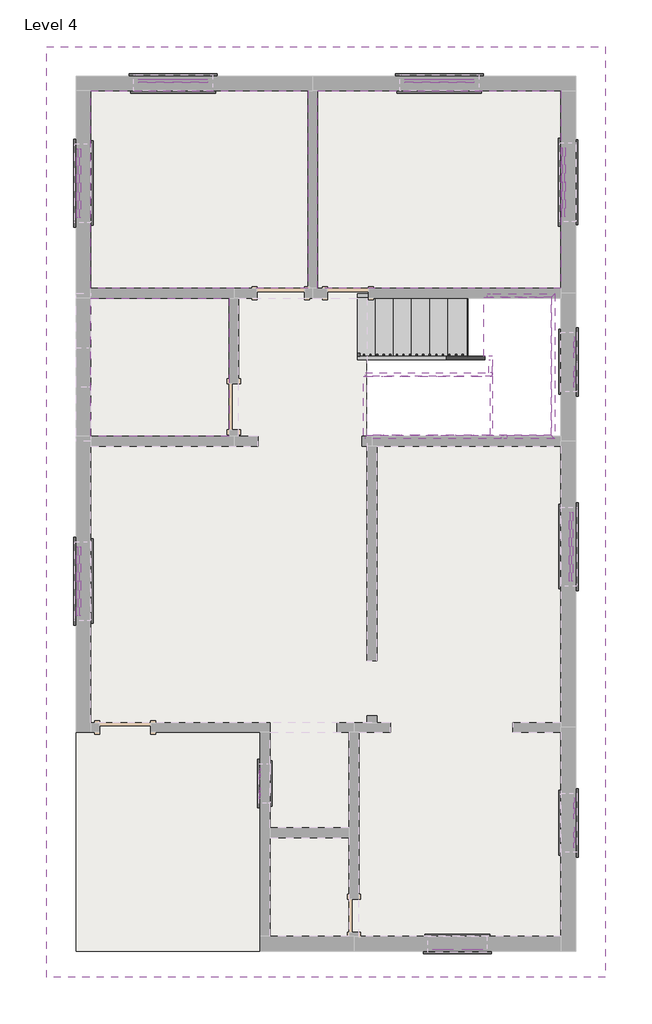
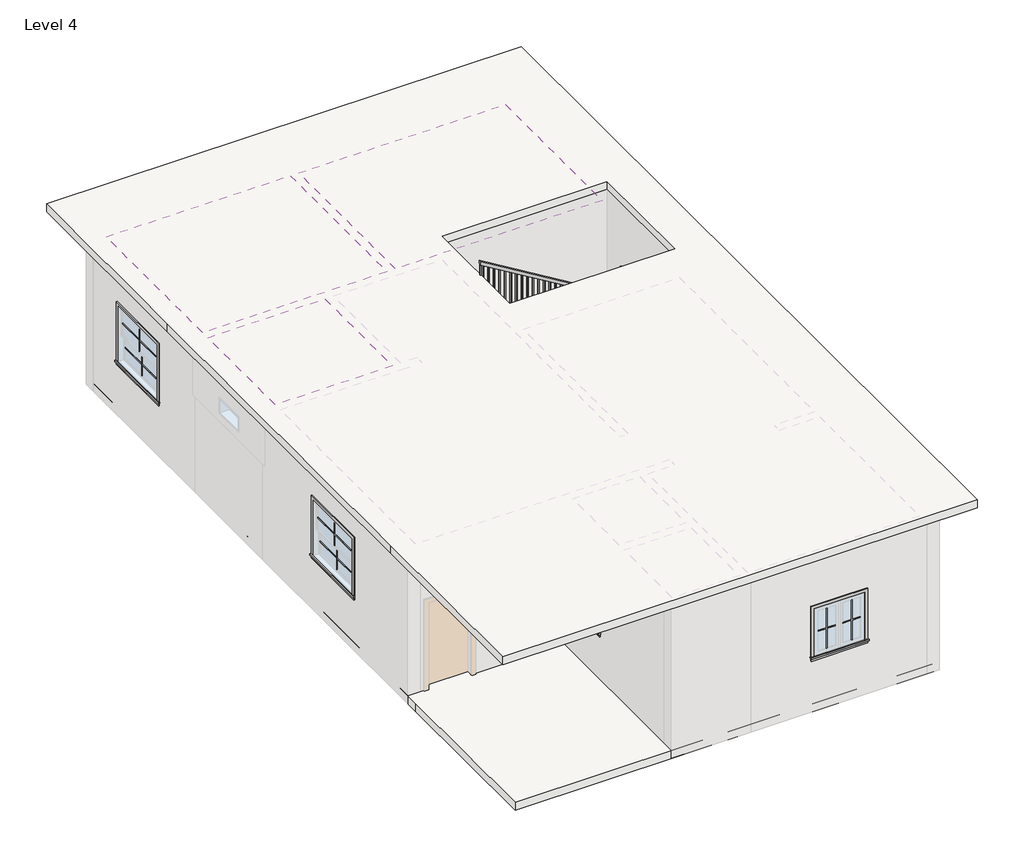
# One storey, part 2 of 2: 40 proxies, 8 members, 3 coverings, 3 slabs, 2 stair flights, 1 railing.
"""IFC4 building model written with IfcOpenShell, lengths in millimetres."""

from ifc_helpers import new_model, si_unit, frame, origin, place, context, project, spatial, polyline, outline, extrude, faceted_brep, transform, mapped, element, save
from components import muntin_pattern_2x2_muntin_pattern_2x2_8b3f23e7, muntin_pattern_2x2_muntin_pattern_2x2_5e52a1c6, muntin_pattern_2x2_muntin_pattern_2x2_d1c6e638, muntin_pattern_2x2_muntin_pattern_2x2_37b95fb2, muntin_pattern_2x2_muntin_pattern_2x2_53152e2c, muntin_pattern_2x2_muntin_pattern_2x2_e8f3e573, trim_window_exterior_flat_with_sill_f44f30ad, trim_window_exterior_flat_with_sill_e2e7eb1d, trim_window_exterior_flat_with_sill_84e24481, trim_window_exterior_flat_with_sill_a665a915, trim_window_interior_flat_picture_frame_1dce1945, trim_window_interior_flat_picture_frame_a40cb921, trim_window_interior_flat_picture_frame_28d4e5dc, trim_window_interior_flat_picture_frame_d485c387, non_monolithic_landing_28d2b2aa, stair_flight_33a07897, stair_flight_2b211656

model = new_model("IFC4")

# Units and contexts
model_context = context("Model", 3, world=origin())
ifc_project = project(units=[si_unit("LENGTHUNIT", "METRE", prefix="MILLI")], contexts=[model_context])

# Site, building, storey
site = spatial("IfcSite", under=ifc_project)
building = spatial("IfcBuilding", under=site)
storey = spatial("IfcBuildingStorey", under=building, Name="Level 4", Elevation=9601.2)

# Proxies
placement = place(None, origin())
muntin_pattern_2x2_muntin_pattern_2x2_shape = muntin_pattern_2x2_muntin_pattern_2x2_8b3f23e7(model_context)
element("IfcBuildingElementProxy", 1, Name="Muntin Pattern_2x2 : Muntin Pattern_2x2", ObjectType="Muntin Pattern_2x2 : Muntin Pattern_2x2", at=placement, inside=storey, context=model_context, shape_type="MappedRepresentation", body=[
    mapped(muntin_pattern_2x2_muntin_pattern_2x2_shape, transform((-5865.439062, 5032.1857363, 11376.025), x_axis=(0.0, 1.0, 0.0), y_axis=(-1.0, 0.0, 0.0), z_axis=(0.0, 0.0, 1.0))),
])
element("IfcBuildingElementProxy", 2, Name="Muntin Pattern_2x2 : Muntin Pattern_2x2", ObjectType="Muntin Pattern_2x2 : Muntin Pattern_2x2", at=placement, inside=storey, context=model_context, shape_type="MappedRepresentation", body=[
    mapped(muntin_pattern_2x2_muntin_pattern_2x2_shape, transform((-5820.989062, 5032.1857363, 10896.6), x_axis=(0.0, 1.0, 0.0), y_axis=(-1.0, 0.0, 0.0), z_axis=(0.0, 0.0, 1.0))),
])
element("IfcBuildingElementProxy", 3, Name="Muntin Pattern_2x2 : Muntin Pattern_2x2", ObjectType="Muntin Pattern_2x2 : Muntin Pattern_2x2", at=placement, inside=storey, context=model_context, shape_type="MappedRepresentation", body=[
    mapped(muntin_pattern_2x2_muntin_pattern_2x2_shape, transform((1786.310938, -581.2142637, 11376.025), x_axis=(0.0, -1.0, 0.0), y_axis=(1.0, 0.0, 0.0), z_axis=(0.0, 0.0, 1.0))),
])
element("IfcBuildingElementProxy", 4, Name="Muntin Pattern_2x2 : Muntin Pattern_2x2", ObjectType="Muntin Pattern_2x2 : Muntin Pattern_2x2", at=placement, inside=storey, context=model_context, shape_type="MappedRepresentation", body=[
    mapped(muntin_pattern_2x2_muntin_pattern_2x2_shape, transform((1741.860938, -581.2142637, 10896.6), x_axis=(0.0, -1.0, 0.0), y_axis=(1.0, 0.0, 0.0), z_axis=(0.0, 0.0, 1.0))),
])
element("IfcBuildingElementProxy", 5, Name="Muntin Pattern_2x2 : Muntin Pattern_2x2", ObjectType="Muntin Pattern_2x2 : Muntin Pattern_2x2", at=placement, inside=storey, context=model_context, shape_type="MappedRepresentation", body=[
    mapped(muntin_pattern_2x2_muntin_pattern_2x2_shape, transform((-5865.439062, -1114.6142637, 11376.025), x_axis=(0.0, 1.0, 0.0), y_axis=(-1.0, 0.0, 0.0), z_axis=(0.0, 0.0, 1.0))),
])
element("IfcBuildingElementProxy", 6, Name="Muntin Pattern_2x2 : Muntin Pattern_2x2", ObjectType="Muntin Pattern_2x2 : Muntin Pattern_2x2", at=placement, inside=storey, context=model_context, shape_type="MappedRepresentation", body=[
    mapped(muntin_pattern_2x2_muntin_pattern_2x2_shape, transform((-5820.989062, -1114.6142637, 10896.6), x_axis=(0.0, 1.0, 0.0), y_axis=(-1.0, 0.0, 0.0), z_axis=(0.0, 0.0, 1.0))),
])
muntin_pattern_2x2_muntin_pattern_2x2_2_shape = muntin_pattern_2x2_muntin_pattern_2x2_5e52a1c6(model_context)
element("IfcBuildingElementProxy", 7, Name="Muntin Pattern_2x2 : Muntin Pattern_2x2", ObjectType="Muntin Pattern_2x2 : Muntin Pattern_2x2", at=placement, inside=storey, context=model_context, shape_type="MappedRepresentation", body=[
    mapped(muntin_pattern_2x2_muntin_pattern_2x2_2_shape, transform((-4401.764062, 6648.2607363, 11376.025), x_axis=(-1.0, 0.0, 0.0), y_axis=(0.0, -1.0, 0.0), z_axis=(0.0, 0.0, 1.0))),
])
element("IfcBuildingElementProxy", 8, Name="Muntin Pattern_2x2 : Muntin Pattern_2x2", ObjectType="Muntin Pattern_2x2 : Muntin Pattern_2x2", at=placement, inside=storey, context=model_context, shape_type="MappedRepresentation", body=[
    mapped(muntin_pattern_2x2_muntin_pattern_2x2_2_shape, transform((-4401.764062, 6603.8107363, 10896.6), x_axis=(-1.0, 0.0, 0.0), y_axis=(0.0, -1.0, 0.0), z_axis=(0.0, 0.0, 1.0))),
])
element("IfcBuildingElementProxy", 9, Name="Muntin Pattern_2x2 : Muntin Pattern_2x2", ObjectType="Muntin Pattern_2x2 : Muntin Pattern_2x2", at=placement, inside=storey, context=model_context, shape_type="MappedRepresentation", body=[
    mapped(muntin_pattern_2x2_muntin_pattern_2x2_2_shape, transform((-286.964062, 6648.2607363, 11376.025), x_axis=(-1.0, 0.0, 0.0), y_axis=(0.0, -1.0, 0.0), z_axis=(0.0, 0.0, 1.0))),
])
element("IfcBuildingElementProxy", 10, Name="Muntin Pattern_2x2 : Muntin Pattern_2x2", ObjectType="Muntin Pattern_2x2 : Muntin Pattern_2x2", at=placement, inside=storey, context=model_context, shape_type="MappedRepresentation", body=[
    mapped(muntin_pattern_2x2_muntin_pattern_2x2_2_shape, transform((-286.964062, 6603.8107363, 10896.6), x_axis=(-1.0, 0.0, 0.0), y_axis=(0.0, -1.0, 0.0), z_axis=(0.0, 0.0, 1.0))),
])
element("IfcBuildingElementProxy", 11, Name="Muntin Pattern_2x2 : Muntin Pattern_2x2", ObjectType="Muntin Pattern_2x2 : Muntin Pattern_2x2", at=placement, inside=storey, context=model_context, shape_type="MappedRepresentation", body=[
    mapped(muntin_pattern_2x2_muntin_pattern_2x2_2_shape, transform((1627.560938, 5044.8857363, 11376.025), x_axis=(0.0, -1.0, 0.0), y_axis=(1.0, 0.0, 0.0), z_axis=(0.0, 0.0, 1.0))),
])
element("IfcBuildingElementProxy", 12, Name="Muntin Pattern_2x2 : Muntin Pattern_2x2", ObjectType="Muntin Pattern_2x2 : Muntin Pattern_2x2", at=placement, inside=storey, context=model_context, shape_type="MappedRepresentation", body=[
    mapped(muntin_pattern_2x2_muntin_pattern_2x2_2_shape, transform((1672.010938, 5044.8857363, 10896.6), x_axis=(0.0, -1.0, 0.0), y_axis=(1.0, 0.0, 0.0), z_axis=(0.0, 0.0, 1.0))),
])
muntin_pattern_2x2_muntin_pattern_2x2_3_shape = muntin_pattern_2x2_muntin_pattern_2x2_d1c6e638(model_context)
element("IfcBuildingElementProxy", 13, Name="Muntin Pattern_2x2 : Muntin Pattern_2x2", ObjectType="Muntin Pattern_2x2 : Muntin Pattern_2x2", at=placement, inside=storey, context=model_context, shape_type="MappedRepresentation", body=[
    mapped(muntin_pattern_2x2_muntin_pattern_2x2_3_shape, transform((1811.710938, -4621.4017637, 10890.25), x_axis=(0.0, -1.0, 0.0), y_axis=(1.0, 0.0, 0.0), z_axis=(0.0, 0.0, 1.0))),
])
element("IfcBuildingElementProxy", 14, Name="Muntin Pattern_2x2 : Muntin Pattern_2x2", ObjectType="Muntin Pattern_2x2 : Muntin Pattern_2x2", at=placement, inside=storey, context=model_context, shape_type="MappedRepresentation", body=[
    mapped(muntin_pattern_2x2_muntin_pattern_2x2_3_shape, transform((219.448438, -6820.0892637, 10890.25), x_axis=(-1.0, 0.0, 0.0), y_axis=(0.0, -1.0, 0.0), z_axis=(0.0, 0.0, 1.0))),
])
element("IfcBuildingElementProxy", 15, Name="Muntin Pattern_2x2 : Muntin Pattern_2x2", ObjectType="Muntin Pattern_2x2 : Muntin Pattern_2x2", at=placement, inside=storey, context=model_context, shape_type="MappedRepresentation", body=[
    mapped(muntin_pattern_2x2_muntin_pattern_2x2_3_shape, transform((1811.710938, 2496.9482363, 10890.25), x_axis=(0.0, -1.0, 0.0), y_axis=(1.0, 0.0, 0.0), z_axis=(0.0, 0.0, 1.0))),
])
muntin_pattern_2x2_muntin_pattern_2x2_4_shape = muntin_pattern_2x2_muntin_pattern_2x2_37b95fb2(model_context)
element("IfcBuildingElementProxy", 16, Name="Muntin Pattern_2x2 : Muntin Pattern_2x2", ObjectType="Muntin Pattern_2x2 : Muntin Pattern_2x2", at=placement, inside=storey, context=model_context, shape_type="MappedRepresentation", body=[
    mapped(muntin_pattern_2x2_muntin_pattern_2x2_4_shape, transform((1811.710938, -5075.4267637, 10890.25), x_axis=(0.0, 1.0, 0.0), y_axis=(-1.0, 0.0, 0.0), z_axis=(0.0, 0.0, 1.0))),
])
element("IfcBuildingElementProxy", 17, Name="Muntin Pattern_2x2 : Muntin Pattern_2x2", ObjectType="Muntin Pattern_2x2 : Muntin Pattern_2x2", at=placement, inside=storey, context=model_context, shape_type="MappedRepresentation", body=[
    mapped(muntin_pattern_2x2_muntin_pattern_2x2_4_shape, transform((-234.576562, -6820.0892637, 10890.25), x_axis=(1.0, 0.0, 0.0), y_axis=(0.0, 1.0, 0.0), z_axis=(0.0, 0.0, 1.0))),
])
element("IfcBuildingElementProxy", 18, Name="Muntin Pattern_2x2 : Muntin Pattern_2x2", ObjectType="Muntin Pattern_2x2 : Muntin Pattern_2x2", at=placement, inside=storey, context=model_context, shape_type="MappedRepresentation", body=[
    mapped(muntin_pattern_2x2_muntin_pattern_2x2_4_shape, transform((1811.710938, 2042.9232363, 10890.25), x_axis=(0.0, 1.0, 0.0), y_axis=(-1.0, 0.0, 0.0), z_axis=(0.0, 0.0, 1.0))),
])
muntin_pattern_2x2_muntin_pattern_2x2_5_shape = muntin_pattern_2x2_muntin_pattern_2x2_53152e2c(model_context)
element("IfcBuildingElementProxy", 19, Name="Muntin Pattern_2x2 : Muntin Pattern_2x2", ObjectType="Muntin Pattern_2x2 : Muntin Pattern_2x2", at=placement, inside=storey, context=model_context, shape_type="MappedRepresentation", body=[
    mapped(muntin_pattern_2x2_muntin_pattern_2x2_5_shape, transform((-3046.039062, -4389.6267637, 10890.25), x_axis=(0.0, 1.0, 0.0), y_axis=(-1.0, 0.0, 0.0), z_axis=(0.0, 0.0, 1.0))),
])
muntin_pattern_2x2_muntin_pattern_2x2_6_shape = muntin_pattern_2x2_muntin_pattern_2x2_e8f3e573(model_context)
element("IfcBuildingElementProxy", 20, Name="Muntin Pattern_2x2 : Muntin Pattern_2x2", ObjectType="Muntin Pattern_2x2 : Muntin Pattern_2x2", at=placement, inside=storey, context=model_context, shape_type="MappedRepresentation", body=[
    mapped(muntin_pattern_2x2_muntin_pattern_2x2_6_shape, transform((-3046.039062, -4088.0017637, 10890.25), x_axis=(0.0, -1.0, 0.0), y_axis=(1.0, 0.0, 0.0), z_axis=(0.0, 0.0, 1.0))),
])
trim_window_exterior_flat_with_sill_shape = trim_window_exterior_flat_with_sill_f44f30ad(model_context)
element("IfcBuildingElementProxy", 21, Name="Trim-Window-Exterior-Flat : with Sill", ObjectType="Trim-Window-Exterior-Flat : with Sill", at=placement, inside=storey, context=model_context, shape_type="MappedRepresentation", body=[
    mapped(trim_window_exterior_flat_with_sill_shape, transform((-5900.364062, 5032.1857363, 11887.2), x_axis=(0.0, -1.0, 0.0), y_axis=(0.0, 0.0, 1.0), z_axis=(-1.0, 0.0, 0.0))),
])
element("IfcBuildingElementProxy", 22, Name="Trim-Window-Exterior-Flat : with Sill", ObjectType="Trim-Window-Exterior-Flat : with Sill", at=placement, inside=storey, context=model_context, shape_type="MappedRepresentation", body=[
    mapped(trim_window_exterior_flat_with_sill_shape, transform((1821.235938, -581.2142637, 11887.2), x_axis=(0.0, 1.0, 0.0), y_axis=(0.0, 0.0, 1.0), z_axis=(1.0, 0.0, 0.0))),
])
element("IfcBuildingElementProxy", 23, Name="Trim-Window-Exterior-Flat : with Sill", ObjectType="Trim-Window-Exterior-Flat : with Sill", at=placement, inside=storey, context=model_context, shape_type="MappedRepresentation", body=[
    mapped(trim_window_exterior_flat_with_sill_shape, transform((-5900.364062, -1114.6142637, 11887.2), x_axis=(0.0, -1.0, 0.0), y_axis=(0.0, 0.0, 1.0), z_axis=(-1.0, 0.0, 0.0))),
])
trim_window_exterior_flat_with_sill_2_shape = trim_window_exterior_flat_with_sill_e2e7eb1d(model_context)
element("IfcBuildingElementProxy", 24, Name="Trim-Window-Exterior-Flat : with Sill", ObjectType="Trim-Window-Exterior-Flat : with Sill", at=placement, inside=storey, context=model_context, shape_type="MappedRepresentation", body=[
    mapped(trim_window_exterior_flat_with_sill_2_shape, transform((-4401.764062, 6683.1857363, 11887.2), x_axis=(1.0, 0.0, 0.0), y_axis=(0.0, 0.0, -1.0), z_axis=(0.0, 1.0, 0.0))),
])
element("IfcBuildingElementProxy", 25, Name="Trim-Window-Exterior-Flat : with Sill", ObjectType="Trim-Window-Exterior-Flat : with Sill", at=placement, inside=storey, context=model_context, shape_type="MappedRepresentation", body=[
    mapped(trim_window_exterior_flat_with_sill_2_shape, transform((-286.964062, 6683.1857363, 11887.2), x_axis=(1.0, 0.0, 0.0), y_axis=(0.0, 0.0, -1.0), z_axis=(0.0, 1.0, 0.0))),
])
element("IfcBuildingElementProxy", 26, Name="Trim-Window-Exterior-Flat : with Sill", ObjectType="Trim-Window-Exterior-Flat : with Sill", at=placement, inside=storey, context=model_context, shape_type="MappedRepresentation", body=[
    mapped(trim_window_exterior_flat_with_sill_2_shape, transform((1592.635938, 5044.8857363, 11887.2), x_axis=(0.0, 1.0, 0.0), y_axis=(0.0, 0.0, -1.0), z_axis=(-1.0, 0.0, 0.0))),
])
trim_window_exterior_flat_with_sill_3_shape = trim_window_exterior_flat_with_sill_84e24481(model_context)
element("IfcBuildingElementProxy", 27, Name="Trim-Window-Exterior-Flat : with Sill", ObjectType="Trim-Window-Exterior-Flat : with Sill", at=placement, inside=storey, context=model_context, shape_type="MappedRepresentation", body=[
    mapped(trim_window_exterior_flat_with_sill_3_shape, transform((1821.235938, -4848.4142637, 11734.8), x_axis=(0.0, 1.0, 0.0), y_axis=(0.0, 0.0, 1.0), z_axis=(1.0, 0.0, 0.0))),
])
element("IfcBuildingElementProxy", 28, Name="Trim-Window-Exterior-Flat : with Sill", ObjectType="Trim-Window-Exterior-Flat : with Sill", at=placement, inside=storey, context=model_context, shape_type="MappedRepresentation", body=[
    mapped(trim_window_exterior_flat_with_sill_3_shape, transform((-7.564062, -6829.6142637, 11734.8), x_axis=(1.0, 0.0, 0.0), y_axis=(0.0, 0.0, 1.0), z_axis=(0.0, -1.0, 0.0))),
])
element("IfcBuildingElementProxy", 29, Name="Trim-Window-Exterior-Flat : with Sill", ObjectType="Trim-Window-Exterior-Flat : with Sill", at=placement, inside=storey, context=model_context, shape_type="MappedRepresentation", body=[
    mapped(trim_window_exterior_flat_with_sill_3_shape, transform((1821.235938, 2269.9357363, 11734.8), x_axis=(0.0, 1.0, 0.0), y_axis=(0.0, 0.0, 1.0), z_axis=(1.0, 0.0, 0.0))),
])
trim_window_exterior_flat_with_sill_4_shape = trim_window_exterior_flat_with_sill_a665a915(model_context)
element("IfcBuildingElementProxy", 30, Name="Trim-Window-Exterior-Flat : with Sill", ObjectType="Trim-Window-Exterior-Flat : with Sill", at=placement, inside=storey, context=model_context, shape_type="MappedRepresentation", body=[
    mapped(trim_window_exterior_flat_with_sill_4_shape, transform((-3055.564062, -4238.8142637, 11734.8), x_axis=(0.0, -1.0, 0.0), y_axis=(0.0, 0.0, 1.0), z_axis=(-1.0, 0.0, 0.0))),
])
trim_window_interior_flat_picture_frame_shape = trim_window_interior_flat_picture_frame_1dce1945(model_context)
element("IfcBuildingElementProxy", 31, Name="Trim-Window-Interior-Flat : Picture Frame", ObjectType="Trim-Window-Interior-Flat : Picture Frame", at=placement, inside=storey, context=model_context, shape_type="MappedRepresentation", body=[
    mapped(trim_window_interior_flat_picture_frame_shape, transform((-5671.764062, 5032.1857363, 11887.2), x_axis=(0.0, 1.0, 0.0), y_axis=(0.0, 0.0, 1.0), z_axis=(1.0, 0.0, 0.0))),
])
element("IfcBuildingElementProxy", 32, Name="Trim-Window-Interior-Flat : Picture Frame", ObjectType="Trim-Window-Interior-Flat : Picture Frame", at=placement, inside=storey, context=model_context, shape_type="MappedRepresentation", body=[
    mapped(trim_window_interior_flat_picture_frame_shape, transform((1592.635938, -581.2142637, 11887.2), x_axis=(0.0, -1.0, 0.0), y_axis=(0.0, 0.0, 1.0), z_axis=(-1.0, 0.0, 0.0))),
])
element("IfcBuildingElementProxy", 33, Name="Trim-Window-Interior-Flat : Picture Frame", ObjectType="Trim-Window-Interior-Flat : Picture Frame", at=placement, inside=storey, context=model_context, shape_type="MappedRepresentation", body=[
    mapped(trim_window_interior_flat_picture_frame_shape, transform((-5671.764062, -1114.6142637, 11887.2), x_axis=(0.0, 1.0, 0.0), y_axis=(0.0, 0.0, 1.0), z_axis=(1.0, 0.0, 0.0))),
])
trim_window_interior_flat_picture_frame_2_shape = trim_window_interior_flat_picture_frame_a40cb921(model_context)
element("IfcBuildingElementProxy", 34, Name="Trim-Window-Interior-Flat : Picture Frame", ObjectType="Trim-Window-Interior-Flat : Picture Frame", at=placement, inside=storey, context=model_context, shape_type="MappedRepresentation", body=[
    mapped(trim_window_interior_flat_picture_frame_2_shape, transform((-4401.764062, 6454.5857363, 11887.2), x_axis=(-1.0, 0.0, 0.0), y_axis=(0.0, 0.0, -1.0), z_axis=(0.0, -1.0, 0.0))),
])
element("IfcBuildingElementProxy", 35, Name="Trim-Window-Interior-Flat : Picture Frame", ObjectType="Trim-Window-Interior-Flat : Picture Frame", at=placement, inside=storey, context=model_context, shape_type="MappedRepresentation", body=[
    mapped(trim_window_interior_flat_picture_frame_2_shape, transform((-286.964062, 6454.5857363, 11887.2), x_axis=(-1.0, 0.0, 0.0), y_axis=(0.0, 0.0, -1.0), z_axis=(0.0, -1.0, 0.0))),
])
element("IfcBuildingElementProxy", 36, Name="Trim-Window-Interior-Flat : Picture Frame", ObjectType="Trim-Window-Interior-Flat : Picture Frame", at=placement, inside=storey, context=model_context, shape_type="MappedRepresentation", body=[
    mapped(trim_window_interior_flat_picture_frame_2_shape, transform((1821.235938, 5044.8857363, 11887.2), x_axis=(0.0, -1.0, 0.0), y_axis=(0.0, 0.0, -1.0), z_axis=(1.0, 0.0, 0.0))),
])
trim_window_interior_flat_picture_frame_3_shape = trim_window_interior_flat_picture_frame_28d4e5dc(model_context)
element("IfcBuildingElementProxy", 37, Name="Trim-Window-Interior-Flat : Picture Frame", ObjectType="Trim-Window-Interior-Flat : Picture Frame", at=placement, inside=storey, context=model_context, shape_type="MappedRepresentation", body=[
    mapped(trim_window_interior_flat_picture_frame_3_shape, transform((1592.635938, -4848.4142637, 11734.8), x_axis=(0.0, -1.0, 0.0), y_axis=(0.0, 0.0, 1.0), z_axis=(-1.0, 0.0, 0.0))),
])
element("IfcBuildingElementProxy", 38, Name="Trim-Window-Interior-Flat : Picture Frame", ObjectType="Trim-Window-Interior-Flat : Picture Frame", at=placement, inside=storey, context=model_context, shape_type="MappedRepresentation", body=[
    mapped(trim_window_interior_flat_picture_frame_3_shape, transform((-7.564062, -6601.0142637, 11734.8), x_axis=(-1.0, 0.0, 0.0), y_axis=(0.0, 0.0, 1.0), z_axis=(0.0, 1.0, 0.0))),
])
element("IfcBuildingElementProxy", 39, Name="Trim-Window-Interior-Flat : Picture Frame", ObjectType="Trim-Window-Interior-Flat : Picture Frame", at=placement, inside=storey, context=model_context, shape_type="MappedRepresentation", body=[
    mapped(trim_window_interior_flat_picture_frame_3_shape, transform((1592.635938, 2269.9357363, 11734.8), x_axis=(0.0, -1.0, 0.0), y_axis=(0.0, 0.0, 1.0), z_axis=(-1.0, 0.0, 0.0))),
])
trim_window_interior_flat_picture_frame_4_shape = trim_window_interior_flat_picture_frame_d485c387(model_context)
element("IfcBuildingElementProxy", 40, Name="Trim-Window-Interior-Flat : Picture Frame", ObjectType="Trim-Window-Interior-Flat : Picture Frame", at=placement, inside=storey, context=model_context, shape_type="MappedRepresentation", body=[
    mapped(trim_window_interior_flat_picture_frame_4_shape, transform((-2903.164062, -4238.8142637, 11734.8), x_axis=(0.0, 1.0, 0.0), y_axis=(0.0, 0.0, 1.0), z_axis=(1.0, 0.0, 0.0))),
])

# Coverings
element("IfcCovering", 41, ObjectType="2' x 4' ACT System", at=placement, inside=storey, context=model_context, shape_type="SweptSolid", body=[
    extrude(outline(polyline([(-5671.764062, 3406.5857363), (-5671.764062, 6454.5857363), (-2318.964062, 6454.5857363), (-2318.964062, 3406.5857363), (-3461.964062, 3406.5857363), (-5671.764062, 3406.5857363)])), frame((0.0, 0.0, 12649.2), z_axis=(0.0, 0.0, 1.0), x_axis=(1.0, 0.0, 0.0)), (0.0, 0.0, 1.0), 57.15),
])
element("IfcCovering", 42, ObjectType="2' x 4' ACT System", at=placement, inside=storey, context=model_context, shape_type="SweptSolid", body=[
    extrude(outline(polyline([(1592.635938, 6454.5857363), (1592.635938, 3406.5857363), (-2166.564062, 3406.5857363), (-2166.564062, 6454.5857363), (1592.635938, 6454.5857363)])), frame((0.0, 0.0, 12649.2), z_axis=(0.0, 0.0, 1.0), x_axis=(1.0, 0.0, 0.0)), (0.0, 0.0, 1.0), 57.15),
])
element("IfcCovering", 43, ObjectType="2' x 4' ACT System", at=placement, inside=storey, context=model_context, shape_type="SweptSolid", body=[
    extrude(outline(polyline([(-5671.764062, 1120.5857363), (-5671.764062, 3254.1857363), (-3538.164062, 3254.1857363), (-3538.164062, 1120.5857363), (-5671.764062, 1120.5857363)])), frame((0.0, 0.0, 12649.2), z_axis=(0.0, 0.0, 1.0), x_axis=(1.0, 0.0, 0.0)), (0.0, 0.0, 1.0), 57.15),
])

# Members
element("IfcMember", 44, ObjectType="Stringer - 2\" Width", at=placement, inside=storey, context=model_context, shape_type="SweptSolid", body=[
    extrude(outline(polyline([(9965.714512, -1552.2130387), (9753.6, -1552.2130387), (9753.6, -1314.127527), (10879.6666667, 543.882473), (11184.4666667, 458.7280165), (9965.714512, -1552.2130387)])), frame((0.0, 3268.950634, 0.0), z_axis=(0.0, 1.0, 0.0), x_axis=(0.0, 0.0, 1.0)), (0.0, 0.0, 1.0), 50.8),
])
element("IfcMember", 45, ObjectType="Stringer - 2\" Width", at=placement, inside=storey, context=model_context, shape_type="SweptSolid", body=[
    extrude(outline(polyline([(9965.714512, -1552.2130387), (9753.6, -1552.2130387), (9753.6, -1314.127527), (10871.6087807, 530.5869613), (11184.4666667, 530.5869613), (11184.4666667, 458.7280165), (9965.714512, -1552.2130387)])), frame((0.0, 2303.750634, 0.0), z_axis=(0.0, 1.0, 0.0), x_axis=(0.0, 0.0, 1.0)), (0.0, 0.0, 1.0), 50.8),
])
element("IfcMember", 46, ObjectType="Stringer - 2\" Width", at=placement, inside=storey, context=model_context, shape_type="SweptSolid", body=[
    extrude(outline(polyline([(10879.6666667, 669.6914495), (11184.4666667, 754.845906), (12505.714512, -1425.2130387), (12149.3057504, -1425.2130387), (10879.6666667, 669.6914495)])), frame((0.0, 1084.550634, 0.0), z_axis=(0.0, 1.0, 0.0), x_axis=(0.0, 0.0, 1.0)), (0.0, 0.0, 1.0), 50.8),
])
element("IfcMember", 47, ObjectType="Stringer - 2\" Width", at=placement, inside=storey, context=model_context, shape_type="SweptSolid", body=[
    extrude(outline(polyline([(10963.9724171, 530.5869613), (11320.3811786, 530.5869613), (12505.714512, -1425.2130387), (12149.3057504, -1425.2130387), (10963.9724171, 530.5869613)])), frame((0.0, 2049.750634, 0.0), z_axis=(0.0, 1.0, 0.0), x_axis=(0.0, 0.0, 1.0)), (0.0, 0.0, 1.0), 50.8),
])
element("IfcMember", 48, ObjectType="Stringer - 2\" Width", at=placement, inside=storey, context=model_context, shape_type="Brep", body=[
    faceted_brep([(754.845906, 1135.350634, 11184.4666667), (754.845906, 1084.550634, 11184.4666667), (1495.7869613, 1084.550634, 11184.4666667), (1444.9869613, 1135.350634, 11184.4666667), (669.6914495, 1135.350634, 10879.6666667), (1444.9869613, 1135.350634, 10879.6666667), (669.6914495, 1084.550634, 10879.6666667), (1495.7869613, 1084.550634, 10879.6666667)], [[[0, 1, 2, 3]], [[4, 0, 3, 5]], [[6, 4, 5, 7]], [[1, 6, 7, 2]], [[1, 0, 4, 6]], [[2, 7, 5, 3]]]),
])
element("IfcMember", 49, ObjectType="Stringer - 2\" Width", at=placement, inside=storey, context=model_context, shape_type="SweptSolid", body=[
    extrude(outline(polyline([(1495.7869613, 1084.550634), (1444.9869613, 1135.350634), (1444.9869613, 3268.950634), (1495.7869613, 3319.750634), (1495.7869613, 1084.550634)])), frame((0.0, 0.0, 10879.6666667), z_axis=(0.0, 0.0, 1.0), x_axis=(1.0, 0.0, 0.0)), (0.0, 0.0, 1.0), 304.8),
])
element("IfcMember", 50, ObjectType="Stringer - 2\" Width", at=placement, inside=storey, context=model_context, shape_type="Brep", body=[
    faceted_brep([(1444.9869613, 3268.950634, 11184.4666667), (1495.7869613, 3319.750634, 11184.4666667), (458.7280165, 3319.750634, 11184.4666667), (458.7280165, 3268.950634, 11184.4666667), (1444.9869613, 3268.950634, 10879.6666667), (543.882473, 3268.950634, 10879.6666667), (1495.7869613, 3319.750634, 10879.6666667), (543.882473, 3319.750634, 10879.6666667)], [[[0, 1, 2, 3]], [[4, 0, 3, 5]], [[6, 4, 5, 7]], [[1, 6, 7, 2]], [[1, 0, 4, 6]], [[2, 7, 5, 3]]]),
])
element("IfcMember", 51, ObjectType="Stringer - 2\" Width", at=placement, inside=storey, context=model_context, shape_type="SweptSolid", body=[
    extrude(outline(polyline([(479.7869613, 2303.750634), (530.5869613, 2303.750634), (530.5869613, 2100.550634), (479.7869613, 2100.550634), (479.7869613, 2303.750634)])), frame((0.0, 0.0, 10879.6666667), z_axis=(0.0, 0.0, 1.0), x_axis=(1.0, 0.0, 0.0)), (0.0, 0.0, 1.0), 304.8),
])

# Railing
element("IfcRailing", 52, ObjectType="Handrail - Rectangular", at=placement, inside=storey, context=model_context, shape_type="SolidModel", body=[
    faceted_brep([(-1552.2130387, 2405.350634, 10837.3333333), (-1552.2130387, 2405.350634, 10777.9318731), (-1552.2130387, 2354.550634, 10777.9318731), (-1552.2130387, 2354.550634, 10837.3333333), (403.5869613, 2405.350634, 12022.6666667), (417.7793707, 2405.350634, 11971.8666667), (417.7793707, 2354.550634, 11971.8666667), (403.5869613, 2354.550634, 12022.6666667), (581.3869613, 2405.350634, 12022.6666667), (581.3869613, 2405.350634, 11971.8666667), (530.5869613, 2354.550634, 11971.8666667), (530.5869613, 2354.550634, 12022.6666667), (581.3869613, 2125.950634, 12022.6666667), (581.3869613, 2075.150634, 11971.8666667), (530.5869613, 2075.150634, 11971.8666667), (530.5869613, 2125.950634, 12022.6666667), (581.3869613, 2125.950634, 12238.1818182), (581.3869613, 2075.150634, 12187.3818182), (530.5869613, 2075.150634, 12187.3818182), (530.5869613, 2125.950634, 12238.1818182), (581.3869613, 1998.950634, 12238.1818182), (581.3869613, 1998.950634, 12187.3818182), (530.5869613, 2049.750634, 12187.3818182), (530.5869613, 2049.750634, 12238.1818182), (454.3869613, 1998.950634, 12238.1818182), (440.1945519, 1998.950634, 12187.3818182), (440.1945519, 2049.750634, 12187.3818182), (454.3869613, 2049.750634, 12238.1818182), (-1425.2130387, 1998.950634, 13377.3333333), (-1425.2130387, 2049.750634, 13377.3333333), (-1425.2130387, 2049.750634, 13317.9318731), (-1425.2130387, 1998.950634, 13317.9318731)], [[[0, 1, 2, 3]], [[1, 0, 4, 5]], [[2, 1, 5, 6]], [[3, 2, 6, 7]], [[0, 3, 7, 4]], [[5, 4, 8, 9]], [[6, 5, 9, 10]], [[7, 6, 10, 11]], [[4, 7, 11, 8]], [[9, 8, 12, 13]], [[10, 9, 13, 14]], [[11, 10, 14, 15]], [[8, 11, 15, 12]], [[13, 12, 16, 17]], [[14, 13, 17, 18]], [[15, 14, 18, 19]], [[12, 15, 19, 16]], [[17, 16, 20, 21]], [[18, 17, 21, 22]], [[19, 18, 22, 23]], [[16, 19, 23, 20]], [[21, 20, 24, 25]], [[22, 21, 25, 26]], [[23, 22, 26, 27]], [[20, 23, 27, 24]], [[28, 29, 30, 31]], [[25, 24, 28, 31]], [[26, 25, 31, 30]], [[27, 26, 30, 29]], [[24, 27, 29, 28]]]),
    extrude(outline(polyline([(13281.371267, -1364.8880387), (13292.9167216, -1383.9380387), (12293.6, -1383.9380387), (12293.6, -1364.8880387), (13281.371267, -1364.8880387)])), frame((0.0, 2014.825634, 0.0), z_axis=(0.0, 1.0, 0.0), x_axis=(0.0, 0.0, 1.0)), (0.0, 0.0, 1.0), 19.05),
    extrude(outline(polyline([(13219.7955094, -1263.2880387), (13231.340964, -1282.3380387), (12293.6, -1282.3380387), (12293.6, -1263.2880387), (13219.7955094, -1263.2880387)])), frame((0.0, 2014.825634, 0.0), z_axis=(0.0, 1.0, 0.0), x_axis=(0.0, 0.0, 1.0)), (0.0, 0.0, 1.0), 19.05),
    extrude(outline(polyline([(13158.2197519, -1161.6880387), (13169.7652064, -1180.7380387), (12293.6, -1180.7380387), (12293.6, -1161.6880387), (13158.2197519, -1161.6880387)])), frame((0.0, 2014.825634, 0.0), z_axis=(0.0, 1.0, 0.0), x_axis=(0.0, 0.0, 1.0)), (0.0, 0.0, 1.0), 19.05),
    extrude(outline(polyline([(13096.6439943, -1060.0880387), (13108.1894488, -1079.1380387), (12124.2666667, -1079.1380387), (12124.2666667, -1060.0880387), (13096.6439943, -1060.0880387)])), frame((0.0, 2014.825634, 0.0), z_axis=(0.0, 1.0, 0.0), x_axis=(0.0, 0.0, 1.0)), (0.0, 0.0, 1.0), 19.05),
    extrude(outline(polyline([(13035.0682367, -958.4880387), (13046.6136913, -977.5380387), (12124.2666667, -977.5380387), (12124.2666667, -958.4880387), (13035.0682367, -958.4880387)])), frame((0.0, 2014.825634, 0.0), z_axis=(0.0, 1.0, 0.0), x_axis=(0.0, 0.0, 1.0)), (0.0, 0.0, 1.0), 19.05),
    extrude(outline(polyline([(12973.4924791, -856.8880387), (12985.0379337, -875.9380387), (12124.2666667, -875.9380387), (12124.2666667, -856.8880387), (12973.4924791, -856.8880387)])), frame((0.0, 2014.825634, 0.0), z_axis=(0.0, 1.0, 0.0), x_axis=(0.0, 0.0, 1.0)), (0.0, 0.0, 1.0), 19.05),
    extrude(outline(polyline([(12911.9167216, -755.2880387), (12923.4621761, -774.3380387), (11954.9333333, -774.3380387), (11954.9333333, -755.2880387), (12911.9167216, -755.2880387)])), frame((0.0, 2014.825634, 0.0), z_axis=(0.0, 1.0, 0.0), x_axis=(0.0, 0.0, 1.0)), (0.0, 0.0, 1.0), 19.05),
    extrude(outline(polyline([(12850.340964, -653.6880387), (12861.8864185, -672.7380387), (11954.9333333, -672.7380387), (11954.9333333, -653.6880387), (12850.340964, -653.6880387)])), frame((0.0, 2014.825634, 0.0), z_axis=(0.0, 1.0, 0.0), x_axis=(0.0, 0.0, 1.0)), (0.0, 0.0, 1.0), 19.05),
    extrude(outline(polyline([(12788.7652064, -552.0880387), (12800.310661, -571.1380387), (11785.6, -571.1380387), (11785.6, -552.0880387), (12788.7652064, -552.0880387)])), frame((0.0, 2014.825634, 0.0), z_axis=(0.0, 1.0, 0.0), x_axis=(0.0, 0.0, 1.0)), (0.0, 0.0, 1.0), 19.05),
    extrude(outline(polyline([(12727.1894488, -450.4880387), (12738.7349034, -469.5380387), (11785.6, -469.5380387), (11785.6, -450.4880387), (12727.1894488, -450.4880387)])), frame((0.0, 2014.825634, 0.0), z_axis=(0.0, 1.0, 0.0), x_axis=(0.0, 0.0, 1.0)), (0.0, 0.0, 1.0), 19.05),
    extrude(outline(polyline([(12665.6136913, -348.8880387), (12677.1591458, -367.9380387), (11785.6, -367.9380387), (11785.6, -348.8880387), (12665.6136913, -348.8880387)])), frame((0.0, 2014.825634, 0.0), z_axis=(0.0, 1.0, 0.0), x_axis=(0.0, 0.0, 1.0)), (0.0, 0.0, 1.0), 19.05),
    extrude(outline(polyline([(12604.0379337, -247.2880387), (12615.5833882, -266.3380387), (11616.2666667, -266.3380387), (11616.2666667, -247.2880387), (12604.0379337, -247.2880387)])), frame((0.0, 2014.825634, 0.0), z_axis=(0.0, 1.0, 0.0), x_axis=(0.0, 0.0, 1.0)), (0.0, 0.0, 1.0), 19.05),
    extrude(outline(polyline([(12542.4621761, -145.6880387), (12554.0076307, -164.7380387), (11616.2666667, -164.7380387), (11616.2666667, -145.6880387), (12542.4621761, -145.6880387)])), frame((0.0, 2014.825634, 0.0), z_axis=(0.0, 1.0, 0.0), x_axis=(0.0, 0.0, 1.0)), (0.0, 0.0, 1.0), 19.05),
    extrude(outline(polyline([(12480.8864185, -44.0880387), (12492.4318731, -63.1380387), (11616.2666667, -63.1380387), (11616.2666667, -44.0880387), (12480.8864185, -44.0880387)])), frame((0.0, 2014.825634, 0.0), z_axis=(0.0, 1.0, 0.0), x_axis=(0.0, 0.0, 1.0)), (0.0, 0.0, 1.0), 19.05),
    extrude(outline(polyline([(12419.310661, 57.5119613), (12430.8561155, 38.4619613), (11446.9333333, 38.4619613), (11446.9333333, 57.5119613), (12419.310661, 57.5119613)])), frame((0.0, 2014.825634, 0.0), z_axis=(0.0, 1.0, 0.0), x_axis=(0.0, 0.0, 1.0)), (0.0, 0.0, 1.0), 19.05),
    extrude(outline(polyline([(12357.7349034, 159.1119613), (12369.2803579, 140.0619613), (11446.9333333, 140.0619613), (11446.9333333, 159.1119613), (12357.7349034, 159.1119613)])), frame((0.0, 2014.825634, 0.0), z_axis=(0.0, 1.0, 0.0), x_axis=(0.0, 0.0, 1.0)), (0.0, 0.0, 1.0), 19.05),
    extrude(outline(polyline([(12296.1591458, 260.7119613), (12307.7046004, 241.6619613), (11446.9333333, 241.6619613), (11446.9333333, 260.7119613), (12296.1591458, 260.7119613)])), frame((0.0, 2014.825634, 0.0), z_axis=(0.0, 1.0, 0.0), x_axis=(0.0, 0.0, 1.0)), (0.0, 0.0, 1.0), 19.05),
    extrude(outline(polyline([(12234.5833882, 362.3119613), (12246.1288428, 343.2619613), (11277.6, 343.2619613), (11277.6, 362.3119613), (12234.5833882, 362.3119613)])), frame((0.0, 2014.825634, 0.0), z_axis=(0.0, 1.0, 0.0), x_axis=(0.0, 0.0, 1.0)), (0.0, 0.0, 1.0), 19.05),
    extrude(outline(polyline([(12173.0076307, 463.9119613), (12184.5530852, 444.8619613), (11277.6, 444.8619613), (11277.6, 463.9119613), (12173.0076307, 463.9119613)])), frame((0.0, 2014.825634, 0.0), z_axis=(0.0, 1.0, 0.0), x_axis=(0.0, 0.0, 1.0)), (0.0, 0.0, 1.0), 19.05),
    extrude(outline(polyline([(546.4619613, 2084.675634), (565.5119613, 2084.675634), (565.5119613, 2065.625634), (546.4619613, 2065.625634), (546.4619613, 2084.675634)])), frame((0.0, 0.0, 11108.2666667), z_axis=(0.0, 0.0, 1.0), x_axis=(1.0, 0.0, 0.0)), (0.0, 0.0, 1.0), 1079.1151515),
    extrude(outline(polyline([(546.4619613, 2186.275634), (565.5119613, 2186.275634), (565.5119613, 2167.225634), (546.4619613, 2167.225634), (546.4619613, 2186.275634)])), frame((0.0, 0.0, 11108.2666667), z_axis=(0.0, 0.0, 1.0), x_axis=(1.0, 0.0, 0.0)), (0.0, 0.0, 1.0), 863.6),
    extrude(outline(polyline([(546.4619613, 2287.875634), (565.5119613, 2287.875634), (565.5119613, 2268.825634), (546.4619613, 2268.825634), (546.4619613, 2287.875634)])), frame((0.0, 0.0, 11108.2666667), z_axis=(0.0, 0.0, 1.0), x_axis=(1.0, 0.0, 0.0)), (0.0, 0.0, 1.0), 863.6),
    extrude(outline(polyline([(495.6619613, 2370.425634), (495.6619613, 2389.475634), (514.7119613, 2389.475634), (514.7119613, 2370.425634), (495.6619613, 2370.425634)])), frame((0.0, 0.0, 11108.2666667), z_axis=(0.0, 0.0, 1.0), x_axis=(1.0, 0.0, 0.0)), (0.0, 0.0, 1.0), 863.6),
    extrude(outline(polyline([(11953.6439943, 387.7119613), (11942.0985397, 368.6619613), (10938.9333333, 368.6619613), (10938.9333333, 387.7119613), (11953.6439943, 387.7119613)])), frame((0.0, 2370.425634, 0.0), z_axis=(0.0, 1.0, 0.0), x_axis=(0.0, 0.0, 1.0)), (0.0, 0.0, 1.0), 19.05),
    extrude(outline(polyline([(11892.0682367, 286.1119613), (11880.5227822, 267.0619613), (10938.9333333, 267.0619613), (10938.9333333, 286.1119613), (11892.0682367, 286.1119613)])), frame((0.0, 2370.425634, 0.0), z_axis=(0.0, 1.0, 0.0), x_axis=(0.0, 0.0, 1.0)), (0.0, 0.0, 1.0), 19.05),
    extrude(outline(polyline([(11830.4924791, 184.5119613), (11818.9470246, 165.4619613), (10938.9333333, 165.4619613), (10938.9333333, 184.5119613), (11830.4924791, 184.5119613)])), frame((0.0, 2370.425634, 0.0), z_axis=(0.0, 1.0, 0.0), x_axis=(0.0, 0.0, 1.0)), (0.0, 0.0, 1.0), 19.05),
    extrude(outline(polyline([(11768.9167216, 82.9119613), (11757.371267, 63.8619613), (10769.6, 63.8619613), (10769.6, 82.9119613), (11768.9167216, 82.9119613)])), frame((0.0, 2370.425634, 0.0), z_axis=(0.0, 1.0, 0.0), x_axis=(0.0, 0.0, 1.0)), (0.0, 0.0, 1.0), 19.05),
    extrude(outline(polyline([(11707.340964, -18.6880387), (11695.7955094, -37.7380387), (10769.6, -37.7380387), (10769.6, -18.6880387), (11707.340964, -18.6880387)])), frame((0.0, 2370.425634, 0.0), z_axis=(0.0, 1.0, 0.0), x_axis=(0.0, 0.0, 1.0)), (0.0, 0.0, 1.0), 19.05),
    extrude(outline(polyline([(11645.7652064, -120.2880387), (11634.2197519, -139.3380387), (10769.6, -139.3380387), (10769.6, -120.2880387), (11645.7652064, -120.2880387)])), frame((0.0, 2370.425634, 0.0), z_axis=(0.0, 1.0, 0.0), x_axis=(0.0, 0.0, 1.0)), (0.0, 0.0, 1.0), 19.05),
    extrude(outline(polyline([(11584.1894488, -221.8880387), (11572.6439943, -240.9380387), (10600.2666667, -240.9380387), (10600.2666667, -221.8880387), (11584.1894488, -221.8880387)])), frame((0.0, 2370.425634, 0.0), z_axis=(0.0, 1.0, 0.0), x_axis=(0.0, 0.0, 1.0)), (0.0, 0.0, 1.0), 19.05),
    extrude(outline(polyline([(11522.6136913, -323.4880387), (11511.0682367, -342.5380387), (10600.2666667, -342.5380387), (10600.2666667, -323.4880387), (11522.6136913, -323.4880387)])), frame((0.0, 2370.425634, 0.0), z_axis=(0.0, 1.0, 0.0), x_axis=(0.0, 0.0, 1.0)), (0.0, 0.0, 1.0), 19.05),
    extrude(outline(polyline([(11461.0379337, -425.0880387), (11449.4924791, -444.1380387), (10600.2666667, -444.1380387), (10600.2666667, -425.0880387), (11461.0379337, -425.0880387)])), frame((0.0, 2370.425634, 0.0), z_axis=(0.0, 1.0, 0.0), x_axis=(0.0, 0.0, 1.0)), (0.0, 0.0, 1.0), 19.05),
    extrude(outline(polyline([(11399.4621761, -526.6880387), (11387.9167216, -545.7380387), (10430.9333333, -545.7380387), (10430.9333333, -526.6880387), (11399.4621761, -526.6880387)])), frame((0.0, 2370.425634, 0.0), z_axis=(0.0, 1.0, 0.0), x_axis=(0.0, 0.0, 1.0)), (0.0, 0.0, 1.0), 19.05),
    extrude(outline(polyline([(11337.8864185, -628.2880387), (11326.340964, -647.3380387), (10430.9333333, -647.3380387), (10430.9333333, -628.2880387), (11337.8864185, -628.2880387)])), frame((0.0, 2370.425634, 0.0), z_axis=(0.0, 1.0, 0.0), x_axis=(0.0, 0.0, 1.0)), (0.0, 0.0, 1.0), 19.05),
    extrude(outline(polyline([(11276.310661, -729.8880387), (11264.7652064, -748.9380387), (10261.6, -748.9380387), (10261.6, -729.8880387), (11276.310661, -729.8880387)])), frame((0.0, 2370.425634, 0.0), z_axis=(0.0, 1.0, 0.0), x_axis=(0.0, 0.0, 1.0)), (0.0, 0.0, 1.0), 19.05),
    extrude(outline(polyline([(11214.7349034, -831.4880387), (11203.1894488, -850.5380387), (10261.6, -850.5380387), (10261.6, -831.4880387), (11214.7349034, -831.4880387)])), frame((0.0, 2370.425634, 0.0), z_axis=(0.0, 1.0, 0.0), x_axis=(0.0, 0.0, 1.0)), (0.0, 0.0, 1.0), 19.05),
    extrude(outline(polyline([(11153.1591458, -933.0880387), (11141.6136913, -952.1380387), (10261.6, -952.1380387), (10261.6, -933.0880387), (11153.1591458, -933.0880387)])), frame((0.0, 2370.425634, 0.0), z_axis=(0.0, 1.0, 0.0), x_axis=(0.0, 0.0, 1.0)), (0.0, 0.0, 1.0), 19.05),
    extrude(outline(polyline([(11091.5833882, -1034.6880387), (11080.0379337, -1053.7380387), (10092.2666667, -1053.7380387), (10092.2666667, -1034.6880387), (11091.5833882, -1034.6880387)])), frame((0.0, 2370.425634, 0.0), z_axis=(0.0, 1.0, 0.0), x_axis=(0.0, 0.0, 1.0)), (0.0, 0.0, 1.0), 19.05),
    extrude(outline(polyline([(11030.0076307, -1136.2880387), (11018.4621761, -1155.3380387), (10092.2666667, -1155.3380387), (10092.2666667, -1136.2880387), (11030.0076307, -1136.2880387)])), frame((0.0, 2370.425634, 0.0), z_axis=(0.0, 1.0, 0.0), x_axis=(0.0, 0.0, 1.0)), (0.0, 0.0, 1.0), 19.05),
    extrude(outline(polyline([(10968.4318731, -1237.8880387), (10956.8864185, -1256.9380387), (10092.2666667, -1256.9380387), (10092.2666667, -1237.8880387), (10968.4318731, -1237.8880387)])), frame((0.0, 2370.425634, 0.0), z_axis=(0.0, 1.0, 0.0), x_axis=(0.0, 0.0, 1.0)), (0.0, 0.0, 1.0), 19.05),
    extrude(outline(polyline([(10906.8561155, -1339.4880387), (10895.310661, -1358.5380387), (9922.9333333, -1358.5380387), (9922.9333333, -1339.4880387), (10906.8561155, -1339.4880387)])), frame((0.0, 2370.425634, 0.0), z_axis=(0.0, 1.0, 0.0), x_axis=(0.0, 0.0, 1.0)), (0.0, 0.0, 1.0), 19.05),
    extrude(outline(polyline([(10845.2803579, -1441.0880387), (10833.7349034, -1460.1380387), (9922.9333333, -1460.1380387), (9922.9333333, -1441.0880387), (10845.2803579, -1441.0880387)])), frame((0.0, 2370.425634, 0.0), z_axis=(0.0, 1.0, 0.0), x_axis=(0.0, 0.0, 1.0)), (0.0, 0.0, 1.0), 19.05),
    extrude(outline(polyline([(546.4619613, 2033.875634), (565.5119613, 2033.875634), (565.5119613, 2014.825634), (546.4619613, 2014.825634), (546.4619613, 2033.875634)])), frame((0.0, 0.0, 11108.2666667), z_axis=(0.0, 0.0, 1.0), x_axis=(1.0, 0.0, 0.0)), (0.0, 0.0, 1.0), 1079.1151515),
    extrude(outline(polyline([(546.4619613, 2370.425634), (546.4619613, 2389.475634), (565.5119613, 2389.475634), (565.5119613, 2370.425634), (546.4619613, 2370.425634)])), frame((0.0, 0.0, 11108.2666667), z_axis=(0.0, 0.0, 1.0), x_axis=(1.0, 0.0, 0.0)), (0.0, 0.0, 1.0), 863.6),
    extrude(outline(polyline([(11969.0379337, 413.1119613), (11957.4924791, 394.0619613), (11108.2666667, 394.0619613), (11108.2666667, 413.1119613), (11969.0379337, 413.1119613)])), frame((0.0, 2370.425634, 0.0), z_axis=(0.0, 1.0, 0.0), x_axis=(0.0, 0.0, 1.0)), (0.0, 0.0, 1.0), 19.05),
    extrude(outline(polyline([(13306.3864185, -1406.1630387), (13317.9318731, -1425.2130387), (12293.6, -1425.2130387), (12293.6, -1406.1630387), (13306.3864185, -1406.1630387)])), frame((0.0, 2014.825634, 0.0), z_axis=(0.0, 1.0, 0.0), x_axis=(0.0, 0.0, 1.0)), (0.0, 0.0, 1.0), 19.05),
    extrude(outline(polyline([(10789.4773276, -1533.1630387), (10777.9318731, -1552.2130387), (9922.9333333, -1552.2130387), (9922.9333333, -1533.1630387), (10789.4773276, -1533.1630387)])), frame((0.0, 2370.425634, 0.0), z_axis=(0.0, 1.0, 0.0), x_axis=(0.0, 0.0, 1.0)), (0.0, 0.0, 1.0), 19.05),
])

# Slabs
element("IfcSlab", 53, ObjectType="Generic - 6\"", at=placement, inside=storey, context=model_context, shape_type="SweptSolid", body=[
    extrude(outline(polyline([(-5900.364062, -3685.8766431), (-5900.364062, 3330.3857363), (-5900.364062, 6683.1857363), (1821.235938, 6683.1857363), (1821.235938, -6829.6142637), (-5900.364062, -6829.6142637), (-5900.364062, -3685.8766431)]), holes=[polyline([(-1404.564062, 3254.1857363), (-1404.564062, 1120.5857363), (1592.635938, 1120.5857363), (1592.635938, 3254.1857363), (-1404.564062, 3254.1857363)])]), frame((0.0, 0.0, 9753.6), z_axis=(0.0, 0.0, 1.0), x_axis=(1.0, 0.0, 0.0)), (0.0, 0.0, 1.0), 152.4),
])
element("IfcSlab", 54, ObjectType="Generic - 6\"", at=placement, inside=storey, context=model_context, shape_type="SweptSolid", body=[
    extrude(outline(polyline([(-6357.564062, -3685.8766431), (-6357.564062, 3330.3857363), (-6357.564062, 7140.3857363), (2278.435938, 7140.3857363), (2278.435938, -7236.0142637), (-6357.564062, -7236.0142637), (-6357.564062, -3685.8766431)]), holes=[polyline([(-1404.564062, 3254.1857363), (-1404.564062, 1120.5857363), (1592.635938, 1120.5857363), (1592.635938, 3254.1857363), (-1404.564062, 3254.1857363)])]), frame((0.0, 0.0, 12954.0), z_axis=(0.0, 0.0, 1.0), x_axis=(1.0, 0.0, 0.0)), (0.0, 0.0, 1.0), 152.4),
])
non_monolithic_landing_shape = non_monolithic_landing_28d2b2aa(model_context)
element("IfcSlab", 55, ObjectType="Non-Monolithic Landing", at=placement, inside=storey, context=model_context, shape_type="MappedRepresentation", body=[
    mapped(non_monolithic_landing_shape, transform((0.0, 0.0, 0.0), x_axis=(1.0, 0.0, 0.0), y_axis=(0.0, 1.0, 0.0), z_axis=(0.0, 0.0, 1.0))),
])

# Stair flights
stair_flight_shape = stair_flight_33a07897(model_context)
element("IfcStairFlight", 56, ObjectType="2\" Tread 1\" Nosing 1/4\" Riser", at=placement, inside=storey, context=model_context, shape_type="MappedRepresentation", body=[
    mapped(stair_flight_shape, transform((0.0, 0.0, 0.0), x_axis=(1.0, 0.0, 0.0), y_axis=(0.0, 1.0, 0.0), z_axis=(0.0, 0.0, 1.0))),
])
stair_flight_2_shape = stair_flight_2b211656(model_context)
element("IfcStairFlight", 57, ObjectType="2\" Tread 1\" Nosing 1/4\" Riser", at=placement, inside=storey, context=model_context, shape_type="MappedRepresentation", body=[
    mapped(stair_flight_2_shape, transform((0.0, 0.0, 0.0), x_axis=(1.0, 0.0, 0.0), y_axis=(0.0, 1.0, 0.0), z_axis=(0.0, 0.0, 1.0))),
])

save(model, "model.ifc")

# Revit data of these elements
# Type "Muntin Pattern_2x2 : Muntin Pattern_2x2"
#   Width [instance default] = 4' - 0"
#   Thickness = 0' - 0 1/2"
#   Height [instance default] = 4' - 0"
#   Distance = 0' - 0 3/4"
#   Interior Material [instance default] = none
#   Exterior Material [instance default] = none
#   Default Elevation = 0
# Type "Trim-Window-Exterior-Flat : with Sill"
#   Trim Width = 0' - 2 1/4"
#   Trim Thickness_Picture Frame = 0' - 1 1/4"
#   Trim Thickness_with Sill = 0' - 0 3/4"
#   Sill Thickness = 0' - 1 1/4"
#   Opening Width [instance default] = 2' - 0"
#   Opening Height [instance default] = 3' - 0"
#   Default Elevation = 4' - 0"
#   Sill = yes
#   Picture Frame = no
#   Trim Material [instance default] = none
# Type "Trim-Window-Interior-Flat : Picture Frame"
#   Trim Thickness_Picture Frame = 0' - 1 1/4"
#   Trim Width = 0' - 2 1/4"
#   Trim Thickness_with Sill = 0' - 0 3/4"
#   Sill Thickness = 0' - 1 1/4"
#   Opening Width [instance default] = 2' - 0"
#   Opening Height [instance default] = 3' - 0"
#   Default Elevation = 4' - 0"
#   Sill = no
#   Picture Frame = yes
#   Trim Material [instance default] = none
# Type "2' x 4' ACT System"
#   Assembly Code = "C3030210"
#   built-in parameter 1002203 = 1 (stored number, unit not read)
#   built-in parameter 1002202 = 1 (stored number, unit not read)
#   Layers, outside or top first: 0' - 1 5/8" "Default" (function 1); 0' - 0 5/8" "Acoustic Ceiling Tile 24 x 48" (function 5)
# Type "Handrail - Rectangular"
#   Assembly Code = "C2010400"
#   built-in parameter 1008612 = 0.0416667 (stored number, unit not read)
#   built-in parameter 1008611 = 0.0416667 (stored number, unit not read)
#   built-in parameter 1008609 = 0.333333 (stored number, unit not read)
#   built-in parameter 1008604 = 0.166667 (stored number, unit not read)
#   built-in parameter 1008603 = 0.166667 (stored number, unit not read)
#   Railing Height = 3' - 0"
#   built-in parameter 1008630 = 2
#   built-in parameter 1008610 = 2
#   built-in parameter 1008618 = Baluster - Square : 3/4"
# Type "Generic - 6\""
#   Assembly Code = "B1010"
#   Function = 0
#   Layers, outside or top first: 0' - 6" no material (function 1)
# Elements 1, 2, 3, 4, 5, 6, 7, 8, 9, 10, 11, 12 (IfcBuildingElementProxy, "Muntin Pattern_2x2 : Muntin Pattern_2x2")
#   Width = 3' - 6"
#   Height = 1' - 5 1/8"
#   Interior Material = Wood - Stained
#   Exterior Material = Clad - White
#   Phase Created = New Construction
#   Materials on its faces: "Clad - White", "Wood - Stained"
# Elements 13, 14, 15, 16, 17, 18 (IfcBuildingElementProxy, "Muntin Pattern_2x2 : Muntin Pattern_2x2")
#   Width = 1' - 0 5/8"
#   Height = 2' - 6 1/2"
#   Interior Material = Wood - Stained
#   Exterior Material = Clad - White
#   Phase Created = New Construction
#   Materials on its faces: "Clad - White", "Wood - Stained"
# Elements 19, 20 (IfcBuildingElementProxy, "Muntin Pattern_2x2 : Muntin Pattern_2x2")
#   Width = 0' - 6 5/8"
#   Height = 2' - 6 1/2"
#   Interior Material = Wood - Stained
#   Exterior Material = Clad - White
#   Phase Created = New Construction
#   Materials on its faces: "Clad - White", "Wood - Stained"
# Elements 21, 22, 23, 24, 25, 26 (IfcBuildingElementProxy, "Trim-Window-Exterior-Flat : with Sill")
#   Opening Width = 4' - 0"
#   Opening Height = 3' - 6"
#   Trim Material = Clad - White
#   Phase Created = New Construction
#   Materials on its faces: "Clad - White"
# Elements 27, 28, 29 (IfcBuildingElementProxy, "Trim-Window-Exterior-Flat : with Sill")
#   Opening Width = 3' - 0"
#   Opening Height = 3' - 0"
#   Trim Material = Clad - White
#   Phase Created = New Construction
#   Materials on its faces: "Clad - White"
# Element 30 (IfcBuildingElementProxy, "Trim-Window-Exterior-Flat : with Sill")
#   Opening Width = 2' - 0"
#   Opening Height = 3' - 0"
#   Trim Material = Clad - White
#   Phase Created = New Construction
#   Materials on its faces: "Clad - White"
# Elements 31, 32, 33, 34, 35, 36 (IfcBuildingElementProxy, "Trim-Window-Interior-Flat : Picture Frame")
#   Opening Width = 4' - 0"
#   Opening Height = 3' - 6"
#   Trim Material = Wood - Stained
#   Phase Created = New Construction
#   Materials on its faces: "Wood - Stained"
# Elements 37, 38, 39 (IfcBuildingElementProxy, "Trim-Window-Interior-Flat : Picture Frame")
#   Opening Width = 3' - 0"
#   Opening Height = 3' - 0"
#   Trim Material = Wood - Stained
#   Phase Created = New Construction
#   Materials on its faces: "Wood - Stained"
# Element 40 (IfcBuildingElementProxy, "Trim-Window-Interior-Flat : Picture Frame")
#   Opening Width = 2' - 0"
#   Opening Height = 3' - 0"
#   Trim Material = Wood - Stained
#   Phase Created = New Construction
#   Materials on its faces: "Wood - Stained"
# Elements 41, 42, 43 (IfcCovering, "2' x 4' ACT System")
#   Height Offset From Level = 10' - 0"
#   Phase Created = New Construction
#   Materials on its faces: "Acoustic Ceiling Tile 24 x 48", "Default"
# Elements 44, 45, 46, 47, 48, 49, 50, 51 (IfcMember, "Stringer - 2\" Width")
#   Phase Created = New Construction
# Element 52 (IfcRailing, "Handrail - Rectangular")
#   Phase Created = New Construction
# Element 53 (IfcSlab, "Generic - 6\"")
#   built-in parameter 1001955 = -1.5708 (stored number, unit not read)
#   Height Offset From Level = 1' - 0"
#   Phase Created = New Construction
#   Materials on its faces: "Default Floor", "CREAM", "FLOOR TILES"
# Element 54 (IfcSlab, "Generic - 6\"")
#   built-in parameter 1001955 = -1.5708 (stored number, unit not read)
#   Height Offset From Level = 11' - 6"
#   Phase Created = New Construction
#   Materials on its faces: "LAVENDER WHITE", "Default Floor", "BURGUNDY COLOUR", "FLOOR TILES"
# Element 55 (IfcSlab, "Non-Monolithic Landing")
#   Phase Created = New Construction
#   Materials on its faces: "BURGUNDY COLOUR"
# Elements 56, 57 (IfcStairFlight, "2\" Tread 1\" Nosing 1/4\" Riser")
#   Phase Created = New Construction
#   Materials on its faces: "BURGUNDY COLOUR"
# Materials
#   "Default": colour RGB 127 127 127, transparency 0, Cost = 0
#   "Acoustic Ceiling Tile 24 x 48": class "Generic", colour RGB 229 229 229, transparency 0, Description = "Acoustic Ceiling Tile 24 x 48", Cost = 0
#   "Clad - White": class "Wood", colour RGB 242 242 238, transparency 0, Cost = 0
#   "Wood - Stained": class "Wood", colour RGB 224 178 126, transparency 0, Cost = 0
#   "Default Floor": colour RGB 128 128 128, transparency 0, Cost = 0
#   "CREAM": class "Generic", colour RGB 120 120 120, transparency 0, Cost = 0
#   "FLOOR TILES": class "Generic", colour RGB 120 120 120, transparency 0, Cost = 0
#   "LAVENDER WHITE": class "Generic", colour RGB 120 120 120, transparency 0, Cost = 0
#   "BURGUNDY COLOUR": class "Generic", colour RGB 120 120 120, transparency 0, Cost = 0
